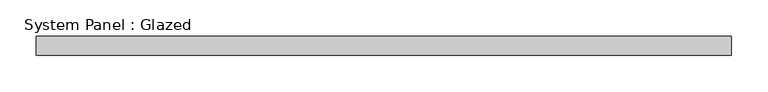
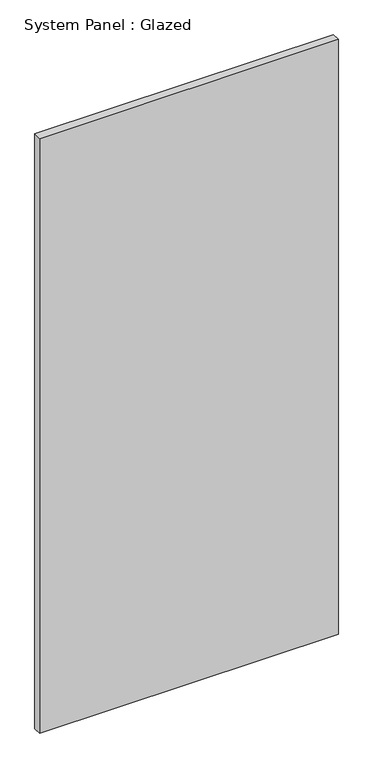
"""IFC4 building model written with IfcOpenShell, lengths in millimetres: plate geometry, System Panel : Glazed."""

from ifc_helpers import new_model, si_unit, origin, origin_with_axes, place, context, project, spatial, polyline, outline, extrude, source, transform, mapped, element, save


def system_panel_glazed_f6d699fe(model_context):
    return source(origin(), model_context, "Body", "SweptSolid", [
        extrude(outline(polyline([(476.25, 19.05), (-476.25, 19.05), (-476.25, 44.45), (476.25, 44.45), (476.25, 19.05)])), origin_with_axes(), (0.0, 0.0, 1.0), 2002.1310998),
    ])


if __name__ == "__main__":
    model = new_model("IFC4")
    model_context = context("Model", 3, world=origin())
    ifc_project = project(units=[si_unit("LENGTHUNIT", "METRE", prefix="MILLI")], contexts=[model_context])
    site = spatial("IfcSite", under=ifc_project)
    building = spatial("IfcBuilding", under=site)
    placement = place(None, origin())
    system_panel_glazed_shape = system_panel_glazed_f6d699fe(model_context)
    element("IfcPlate", 1, ObjectType="System Panel : Glazed", at=placement, inside=building, context=model_context, shape_type="MappedRepresentation", body=[
        mapped(system_panel_glazed_shape, transform((0.0, 0.0, 0.0), x_axis=(1.0, 0.0, 0.0), y_axis=(0.0, 1.0, 0.0), z_axis=(0.0, 0.0, 1.0))),
    ])
    save(model, "model.ifc")

# Revit data of these elements
# Type "System Panel : Glazed"
#   Construction Type Id = "GSP4R"
#   Analytic Construction = "1/8 in Pilkington single glazing"
#   Visual Light Transmittance = 0.9
#   Solar Heat Gain Coefficient = 0.86
#   Heat Transfer Coefficient (U) = 1.18115 BTU/(h·ft²·°F)
#   Define Thermal Properties by = 1
# Element 1 (IfcPlate, "System Panel : Glazed")
#   Materials on its faces: "Glass"
# Materials
#   "Glass": class "Glass", colour RGB 0 128 192, transparency 0.75, Description = "Soda Lime Glass", Cost = 0
